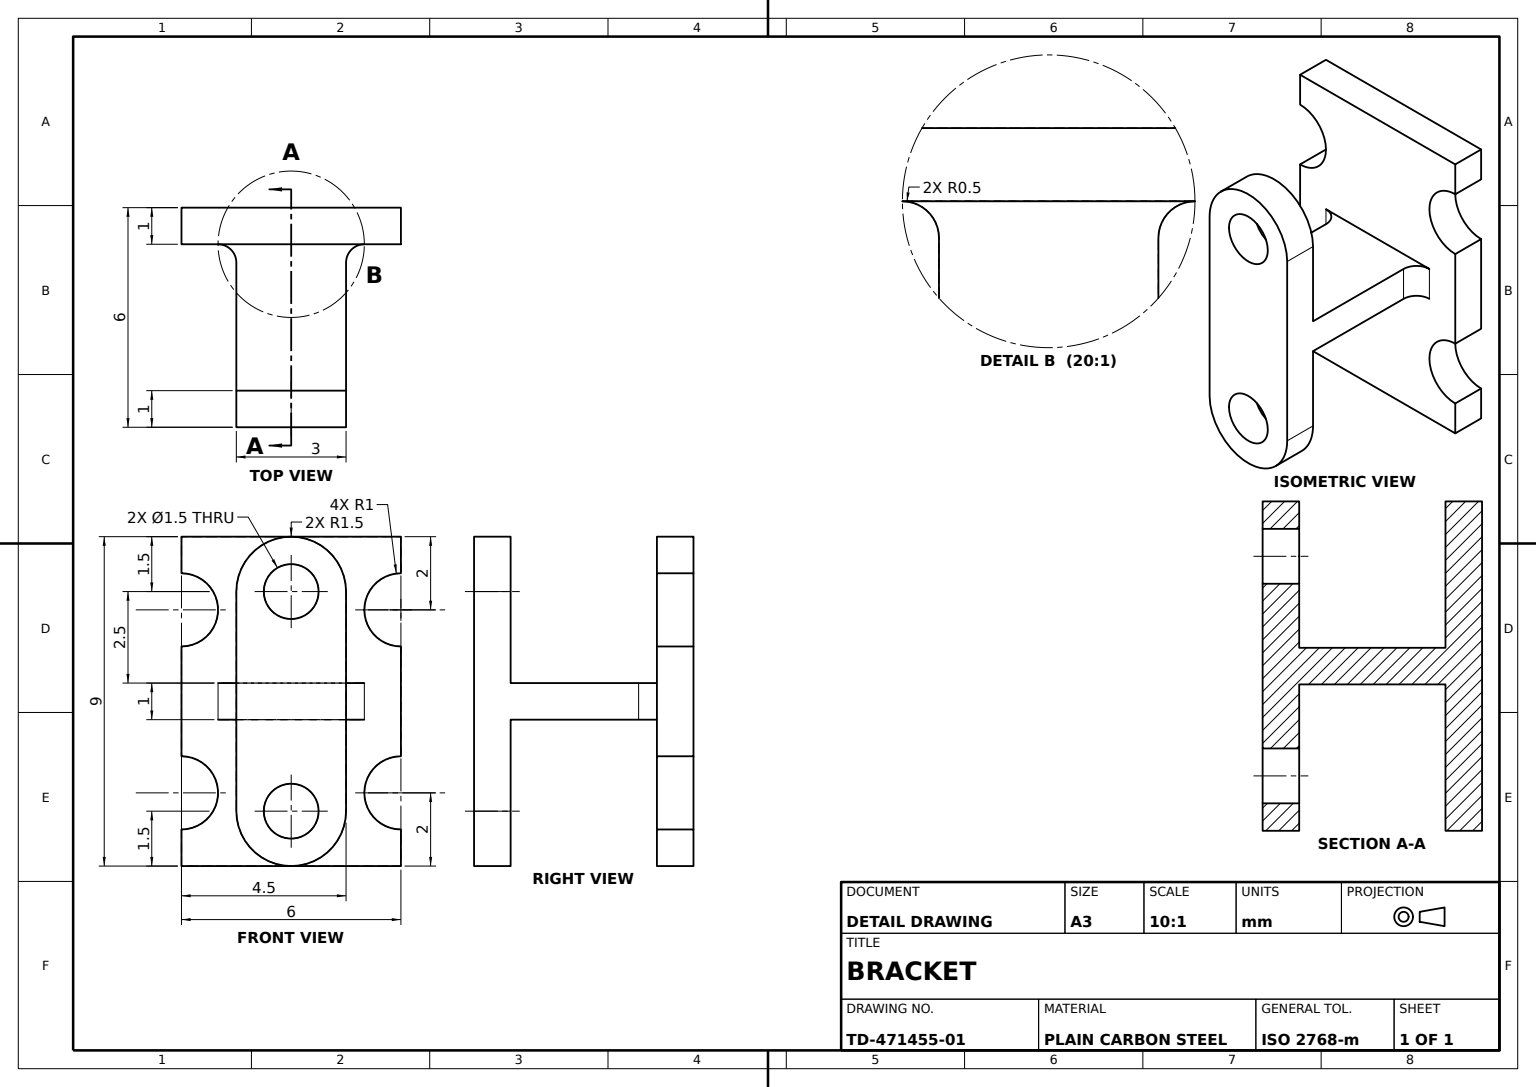
SolidWorks part; units mm, degrees
material "Plain Carbon Steel"
ref_plane "Front Plane" through (0, 0, 0) normal (0, 0, 1) x (1, 0, 0)
ref_plane "Top Plane" through (0, 0, 0) normal (0, 1, 0) x (1, 0, 0)
ref_plane "Right Plane" through (0, 0, 0) normal (1, 0, 0) x (0, 0, -1)
sketch "Base Plate Sketch" plane through (0, 0, 0) normal (0, 0, 1) x (1, 0, 0)
  line L0 (-3, 4.5) -> (3, 4.5)
  line L1 (3, 4.5) -> (3, 3.5)
  line L2 (3, -4.5) -> (3, -3.5)
  line L3 (3, 1.5) -> (3, -1.5)
  line L4 (-3, -4.5) -> (3, -4.5)
  line L5 (0, 5.765) -> (0, -5.0089) construction
  line L6 (-2.832, 0) -> (4.896, 0) construction
  line L7 (-3, -4.5) -> (-3, -3.5)
  line L8 (-3, 1.5) -> (-3, -1.5)
  line L9 (-3, 4.5) -> (-3, 3.5)
  arc A0 (3, 3.5) -> (3, 1.5) centre (3, 2.5) ccw
  arc A1 (3, -3.5) -> (3, -1.5) centre (3, -2.5) cw
  arc A2 (-3, -3.5) -> (-3, -1.5) centre (-3, -2.5) ccw
  arc A3 (-3, 3.5) -> (-3, 1.5) centre (-3, 2.5) cw
  point P12 (3, 0)
  point P19 (0, -4.5)
  point P26 (0, 4.5)
  dimension "D5" = 1
  dimension "D1" = 3
  dimension "D2" = 1
  dimension "D3" = 4.5
  dimension "D4" = 2
  dimension "D6" = 3
extrude "Base Plate" add sketch "Base Plate Sketch" along normal blind 1
sketch "Web Sketch" plane through (0, 0, 1) normal (0, 0, 1) x (1, 0, 0)
  line L1 (-1.5, 0.5) -> (1.5, 0.5)
  line L2 (-1.5, 0.5) -> (-1.5, -0.5)
  line L3 (-1.5, -0.5) -> (1.5, -0.5)
  line L4 (1.5, 0.5) -> (1.5, -0.5)
  line L5 (-1.5, 0.5) -> (1.5, -0.5) construction
  line L6 (-1.5, -0.5) -> (1.5, 0.5) construction
  point P0 (0, 0)
  dimension "D1" = 1
  dimension "D2" = 3
extrude "Web" add sketch "Web Sketch" along normal blind 4
sketch "Lug Sketch" plane through (0, 0, 5) normal (0, 0, 1) x (1, 0, 0)
  line L0 (0, 3) -> (0, -3) construction
  line L1 (1.5, 3) -> (1.5, -3)
  line L2 (-1.5, 3) -> (-1.5, -3)
  line L3 (3, 4.5) -> (-3, 4.5) construction
  line L4 (-3, -4.5) -> (3, -4.5) construction
  arc A0 (1.5, 3) -> (-1.5, 3) centre (0, 3) ccw
  arc A1 (-1.5, -3) -> (1.5, -3) centre (0, -3) ccw
  point P3 (0, 0)
  dimension "D1" = 1.5
extrude "Lug" add sketch "Lug Sketch" along normal blind 1
sketch "Lug Holes Sketch" plane through (0, 0, 6) normal (0, 0, 1) x (1, 0, 0)
  line L0 (1.5, -3) -> (1.5, 3) construction
  line L1 (3, 4.5) -> (-3, 4.5) construction
  line L2 (-3, -4.5) -> (3, -4.5) construction
  circle A0 centre (0, 3) radius 0.75
  circle A1 centre (0, -3) radius 0.75
  dimension "D1" = 1.5
  dimension "D2" = 1.5
  dimension "D3" = 1.5
  dimension "D4" = 1.5
  dimension "D5" = 1.5
  dimension "D6" = 1.5
extrude "Lug Holes 2x" cut sketch "Lug Holes Sketch" against normal blind 1
fillet "Web Fillet R0.5" radius 0.5 2 edges at (1.5, 0, 1) (-1.5, 0, 1)
